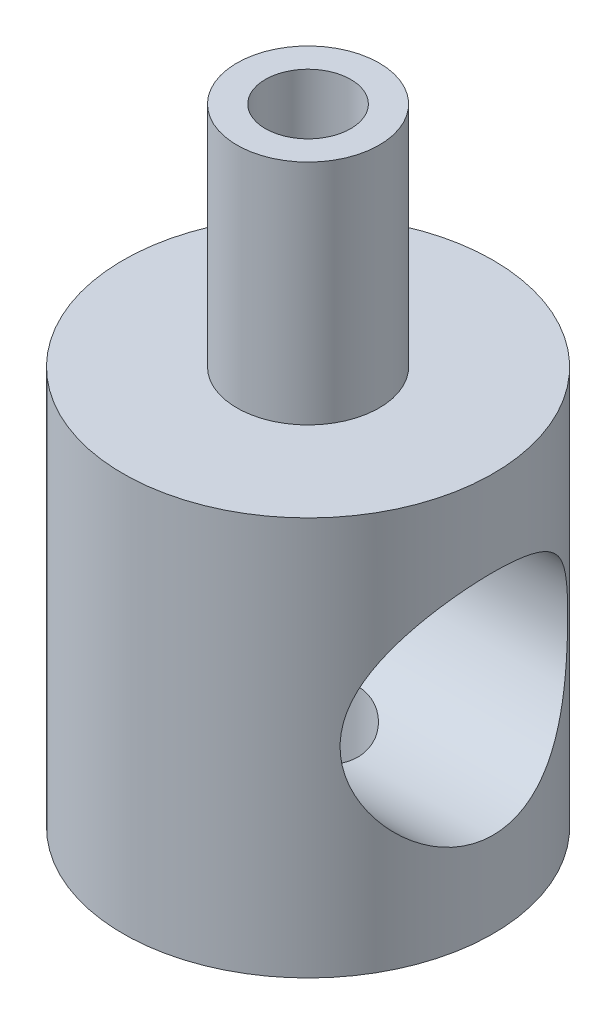
from build123d import *

# Parameters (mm, degrees)
CROSS_HOLE_SKETCH_R     = 4
CROSS_HOLE_8_DEPTH      = 44
NIPPLE_POCKET_SKETCH_R  = 1.75
NIPPLE_POCKET_3_5_DEPTH = 5
CABLE_BORE_SKETCH_R     = 1.5
CABLE_BORE_3_DEPTH      = 13


with BuildPart() as part:
    # Barrel Profile Sketch → Barrel Body Revolve (revolve)
    with BuildSketch(Plane.XY, mode=Mode.PRIVATE) as barrel_body_revolve_sk:
        Polygon((0, 0), (0, 22), (2.5, 22), (2.5, 14), (6.5, 14), (6.5, 0), align=None)
    revolve(barrel_body_revolve_sk.sketch.rotate(Axis((0, 0, 0), (0, 1, 0)), 90), axis=Axis((0, 0, 0), (0, 1, 0)))

    # Cross Hole Sketch → Cross Hole Ø8 (cut, symmetric)
    with BuildSketch(Plane(origin=(0, 0, 0), x_dir=(0, 0, -1), z_dir=(1, 0, 0))):
        with Locations((0, 7)):
            Circle(CROSS_HOLE_SKETCH_R)
    extrude(amount=CROSS_HOLE_8_DEPTH, both=True, mode=Mode.SUBTRACT)

    # Nipple Pocket Sketch → Nipple Pocket Ø3.5 (cut)
    with BuildSketch(Plane.XZ):
        with Locations(Location((0, 0, 0), (0, 0, 270))):
            Circle(NIPPLE_POCKET_SKETCH_R)
    extrude(amount=-NIPPLE_POCKET_3_5_DEPTH, mode=Mode.SUBTRACT)

    # Cable Bore Sketch → Cable Bore Ø3 (cut)
    with BuildSketch(Plane(origin=(0, 22, 0), x_dir=(1, 0, 0), z_dir=(0, 1, 0))):
        with Locations(Location((0, 0, 0), (0, 0, 270))):
            Circle(CABLE_BORE_SKETCH_R)
    extrude(amount=-CABLE_BORE_3_DEPTH, mode=Mode.SUBTRACT)


solid = part.part
